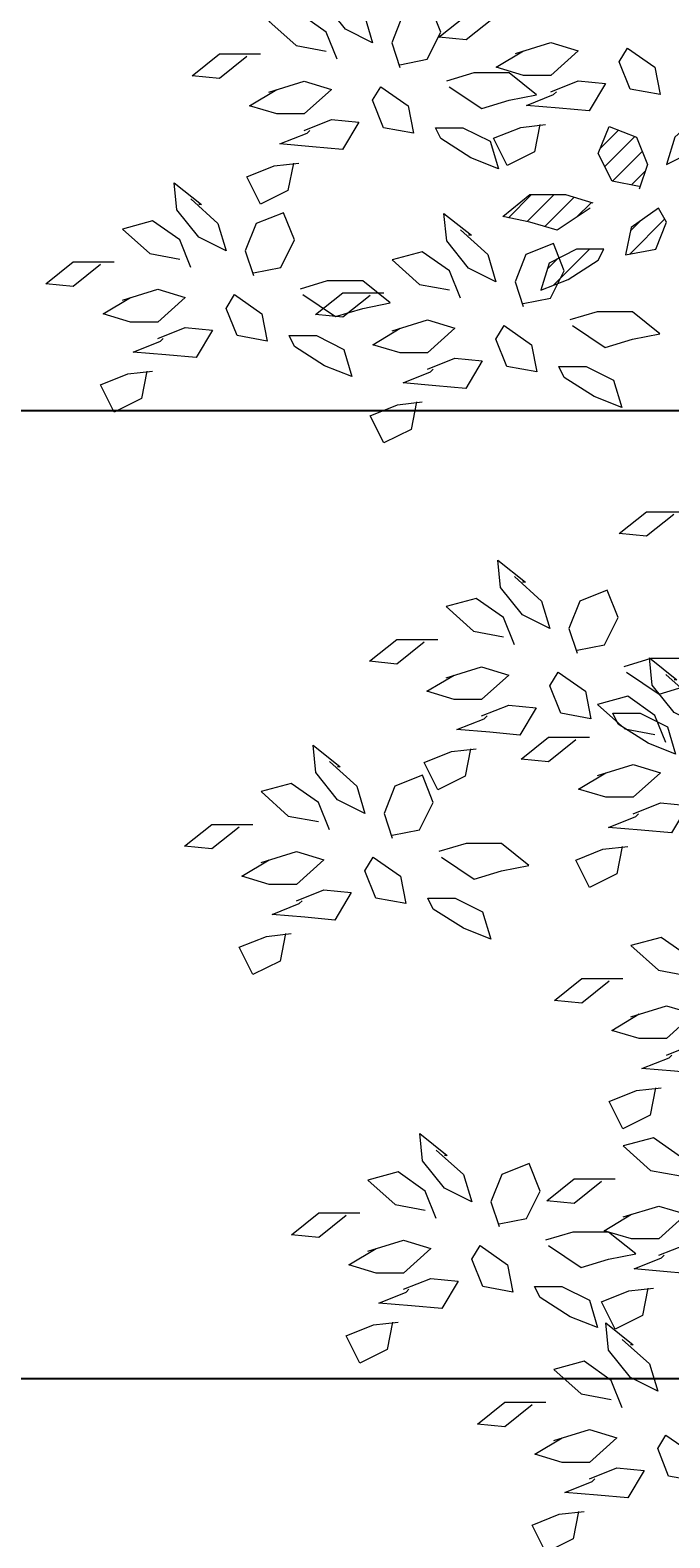
# Model space of a CAD drawing. Units: inches. Extents: x 1770 to 2988, y 1161 to 3221.
# Tile 39 of 44: x 2655 to 2687, y 2750 to 2825. Entities that reach past the tile are written whole.
import ezdxf

# ---------------------------------------------------------------- set-up
doc = ezdxf.new("R2010")
doc.units = ezdxf.units.IN
doc.layers.add('A-ANNO-DIMS', color=2, linetype='Continuous', lineweight=18)
doc.layers.add('trees1', color=250, linetype='Continuous', lineweight=13)
doc.styles.get("Standard").update_dxf_attribs({"font": 'arial.ttf'})
doc.dimstyles.get("Standard").update_dxf_attribs({"dimtxt": 0.18, "dimasz": 0.18, "dimexe": 0.18, "dimexo": 0.0625, "dimgap": 0.09, "dimtad": 0, "dimtih": 1, "dimtoh": 1, "dimdec": 4, "dimzin": 0, "dimdsep": 46, "dimtxsty": 'Standard', "dimcen": 0.09, "dimadec": 0, "dimazin": 0, "dimtfac": 1, "dimtdec": 4, "dimtofl": 0, "dimtmove": 0, "dimatfit": 3, "dimfxl": 1, "dimtolj": 1, "dimtzin": 0, "dimarcsym": 0})

# ---------------------------------------------------------------- blocks, each defined once
blk = doc.blocks.new('*X10')
at = {"color": 0}
for p, q in [((0.5118, -0.9024), (0.54, -0.8742)), ((0.5068, -0.8897), (0.5149, -0.8816))]:
    blk.add_line(p, q, dxfattribs=at)
blk = doc.blocks.new('*X11')
at = {"color": 0}
for p, q in [((0.5716, -0.8779), (0.5992, -0.8504)), ((0.5721, -0.8598), (0.5799, -0.852))]:
    blk.add_line(p, q, dxfattribs=at)
blk = doc.blocks.new('*X12')
at = {"color": 0}
for p, q in [((0.4764, -0.8494), (0.4945, -0.8313)), ((0.4911, -0.8524), (0.5122, -0.8313)), ((0.5049, -0.8563), (0.5279, -0.8333)), ((0.5296, -0.8493), (0.5415, -0.8374))]:
    blk.add_line(p, q, dxfattribs=at)
blk = doc.blocks.new('*X13')
at = {"color": 0}
for p, q in [((0.5486, -0.7949), (0.5629, -0.7806)), ((0.552, -0.8092), (0.5755, -0.7857)), ((0.5582, -0.8207), (0.5814, -0.7974)), ((0.5729, -0.8236), (0.5839, -0.8126))]:
    blk.add_line(p, q, dxfattribs=at)
blk = doc.blocks.new('tree342')
at = {"color": 0}
for points in [[(-770.6, 1840.1), (-749.1, 1820.8), (-742.7, 1799.4), (-764.1, 1810.1), (-781.3, 1831.6), (-783.5, 1853), (-762, 1835.8), (-764.1, 1835.8)], [(-721.2, 1782.2), (-699.7, 1786.5), (-689, 1807.9), (-697.6, 1829.4), (-719.1, 1820.8), (-727.6, 1799.4), (-721.2, 1780)], [(-770.6, 1786.5), (-779.2, 1807.9), (-800.7, 1823), (-824.3, 1816.5), (-802.8, 1797.2), (-779.2, 1792.9)], [(-647.7, 1818.9), (-669.2, 1801.7), (-690.7, 1803.9), (-669.2, 1821), (-637, 1821)], [(-841.5, 1788.6), (-862.9, 1771.5), (-884.4, 1773.6), (-862.9, 1790.8), (-830.7, 1790.8)], [(-630.5, 1791), (-602.6, 1799.6), (-581.1, 1793.1), (-602.6, 1773.8), (-624.1, 1773.8), (-645.6, 1780.3), (-624.1, 1793.1)], [(-824.3, 1760.7), (-796.4, 1769.3), (-774.9, 1762.9), (-796.4, 1743.6), (-817.8, 1743.6), (-839.3, 1750), (-817.8, 1762.9)], [(-682.5, 1765), (-656.8, 1747.9), (-635.3, 1754.3), (-613.8, 1758.6), (-635.3, 1775.8), (-663.2, 1775.8), (-684.7, 1769.3)], [(-602.6, 1760.9), (-581.1, 1769.5), (-559.7, 1767.4), (-572.5, 1745.9), (-596.2, 1748.1), (-621.9, 1750.2), (-600.5, 1758.8), (-598.3, 1760.9)], [(-483.8, 1744.6), (-505.2, 1725.3), (-511.7, 1703.8), (-490.2, 1714.5), (-473, 1736), (-470.9, 1757.5), (-492.4, 1740.3), (-490.2, 1740.3)], [(-796.4, 1730.7), (-774.9, 1739.3), (-753.4, 1737.1), (-766.3, 1715.7), (-789.9, 1717.8), (-815.7, 1720), (-794.2, 1728.5), (-792.1, 1730.7)], [(-611.2, 1735.2), (-615.5, 1713.7), (-637, 1703), (-647.7, 1724.5), (-626.2, 1733), (-606.9, 1735.2)], [(-533.2, 1686.6), (-554.6, 1690.9), (-565.4, 1712.4), (-556.8, 1733.8), (-535.3, 1725.3), (-526.7, 1703.8), (-533.2, 1684.5)], [(-804.9, 1704.9), (-809.2, 1683.5), (-830.7, 1672.7), (-841.5, 1694.2), (-820, 1702.8), (-800.7, 1704.9)], [(-885.6, 1676.8), (-864.2, 1657.5), (-857.7, 1636), (-879.2, 1646.7), (-896.4, 1668.2), (-898.5, 1689.6), (-877, 1672.5), (-879.2, 1672.5)], [(-571.8, 1669.5), (-597.6, 1652.3), (-619.1, 1658.7), (-640.5, 1663), (-619.1, 1680.2), (-591.1, 1680.2), (-569.7, 1673.8)], [(-885.6, 1623.1), (-894.2, 1644.6), (-915.7, 1659.6), (-939.3, 1653.2), (-917.8, 1633.9), (-894.2, 1629.6)], [(-836.2, 1618.8), (-814.8, 1623.1), (-804, 1644.6), (-812.6, 1666), (-834.1, 1657.5), (-842.7, 1636), (-836.2, 1616.7)], [(-673.7, 1652.6), (-652.2, 1633.3), (-645.8, 1611.8), (-667.3, 1622.5), (-684.5, 1644), (-686.6, 1665.4), (-665.1, 1648.3), (-667.3, 1648.3)], [(-673.7, 1598.9), (-682.3, 1620.4), (-703.8, 1635.4), (-727.4, 1629), (-705.9, 1609.6), (-682.3, 1605.4)], [(-624.3, 1594.6), (-602.9, 1598.9), (-592.1, 1620.4), (-600.7, 1641.8), (-622.2, 1633.3), (-630.8, 1611.8), (-624.3, 1592.5)], [(-956.5, 1625.3), (-978, 1608.1), (-999.4, 1610.2), (-978, 1627.4), (-945.8, 1627.4)], [(-797.6, 1601.7), (-771.8, 1584.5), (-750.3, 1590.9), (-728.9, 1595.2), (-750.3, 1612.4), (-778.3, 1612.4), (-799.7, 1606)], [(-939.3, 1597.4), (-911.4, 1606), (-889.9, 1599.5), (-911.4, 1580.2), (-932.9, 1580.2), (-954.3, 1586.6), (-932.9, 1599.5)], [(-744.6, 1601.1), (-766.1, 1583.9), (-787.5, 1586), (-766.1, 1603.2), (-733.8, 1603.2)], [(-585.7, 1577.5), (-559.9, 1560.3), (-538.4, 1566.7), (-517, 1571), (-538.4, 1588.2), (-566.3, 1588.2), (-587.8, 1581.8)], [(-911.4, 1567.3), (-889.9, 1575.9), (-868.4, 1573.8), (-881.3, 1552.3), (-905, 1554.4), (-930.7, 1556.6), (-909.2, 1565.2), (-907.1, 1567.3)], [(-727.4, 1573.2), (-699.5, 1581.8), (-678, 1575.3), (-699.5, 1556), (-721, 1556), (-742.4, 1562.4), (-721, 1575.3)], [(-699.5, 1543.1), (-678, 1551.7), (-656.5, 1549.6), (-669.4, 1528.1), (-693, 1530.2), (-718.8, 1532.4), (-697.3, 1541), (-695.2, 1543.1)], [(-920, 1541.6), (-924.3, 1520.1), (-945.8, 1509.4), (-956.5, 1530.8), (-935, 1539.4), (-915.7, 1541.6)], [(-708.1, 1517.4), (-712.4, 1495.9), (-733.8, 1485.2), (-744.6, 1506.6), (-723.1, 1515.2), (-703.8, 1517.4)], [(-506.1, 1429.1), (-527.6, 1411.9), (-549, 1414.1), (-527.6, 1431.2), (-495.4, 1431.2)], [(-631.3, 1380.3), (-609.9, 1361), (-603.4, 1339.5), (-624.9, 1350.3), (-642.1, 1371.7), (-644.2, 1393.2), (-622.7, 1376), (-624.9, 1376)], [(-631.3, 1326.6), (-639.9, 1348.1), (-661.4, 1363.1), (-685, 1356.7), (-663.5, 1337.4), (-639.9, 1333.1)], [(-581.9, 1322.4), (-560.5, 1326.6), (-549.7, 1348.1), (-558.3, 1369.6), (-579.8, 1361), (-588.4, 1339.5), (-581.9, 1320.2)], [(-702.2, 1328.8), (-723.7, 1311.6), (-745.1, 1313.8), (-723.7, 1330.9), (-691.5, 1330.9)], [(-543.3, 1305.2), (-517.5, 1288), (-496, 1294.5), (-474.6, 1298.7), (-496, 1315.9), (-524, 1315.9), (-545.4, 1309.5)], [(-512.3, 1303.5), (-490.8, 1284.2), (-484.3, 1262.8), (-505.8, 1273.5), (-523, 1294.9), (-525.1, 1316.4), (-503.7, 1299.2), (-505.8, 1299.2)], [(-685, 1300.9), (-657.1, 1309.5), (-635.6, 1303), (-657.1, 1283.7), (-678.6, 1283.7), (-700.1, 1290.2), (-678.6, 1303)], [(-657.1, 1270.9), (-635.6, 1279.4), (-614.2, 1277.3), (-627, 1255.8), (-650.7, 1258), (-676.4, 1260.1), (-655, 1268.7), (-652.8, 1270.9)], [(-512.3, 1249.9), (-520.9, 1271.3), (-542.3, 1286.4), (-566, 1279.9), (-544.5, 1260.6), (-520.9, 1256.3)], [(-776.6, 1235.1), (-755.2, 1215.8), (-748.7, 1194.3), (-770.2, 1205), (-787.4, 1226.5), (-789.5, 1248), (-768.1, 1230.8), (-770.2, 1230.8)], [(-665.7, 1245.1), (-670, 1223.6), (-691.5, 1212.9), (-702.2, 1234.4), (-680.7, 1243), (-661.4, 1245.1)], [(-583.1, 1252), (-604.6, 1234.9), (-626.1, 1237), (-604.6, 1254.2), (-572.4, 1254.2)], [(-566, 1224.1), (-538, 1232.7), (-516.6, 1226.3), (-538, 1207), (-559.5, 1207), (-581, 1213.4), (-559.5, 1226.3)], [(-727.3, 1177.1), (-705.8, 1181.4), (-695, 1202.9), (-703.6, 1224.4), (-725.1, 1215.8), (-733.7, 1194.3), (-727.3, 1175)], [(-776.6, 1181.4), (-785.2, 1202.9), (-806.7, 1217.9), (-830.3, 1211.5), (-808.9, 1192.2), (-785.2, 1187.9)], [(-538, 1194.1), (-516.6, 1202.7), (-495.1, 1200.5), (-508, 1179.1), (-531.6, 1181.2), (-557.4, 1183.3), (-535.9, 1191.9), (-533.7, 1194.1)], [(-847.5, 1183.6), (-869, 1166.4), (-890.5, 1168.6), (-869, 1185.7), (-836.8, 1185.7)], [(-830.3, 1155.7), (-802.4, 1164.3), (-780.9, 1157.8), (-802.4, 1138.5), (-823.9, 1138.5), (-845.4, 1145), (-823.9, 1157.8)], [(-688.6, 1160), (-662.8, 1142.8), (-641.4, 1149.2), (-619.9, 1153.5), (-641.4, 1170.7), (-669.3, 1170.7), (-690.7, 1164.3)], [(-546.6, 1168.3), (-550.9, 1146.9), (-572.4, 1136.1), (-583.1, 1157.6), (-561.7, 1166.2), (-542.3, 1168.3)], [(-802.4, 1125.6), (-780.9, 1134.2), (-759.5, 1132.1), (-772.3, 1110.6), (-796, 1112.8), (-821.7, 1114.9), (-800.3, 1123.5), (-798.1, 1125.6)], [(-811, 1099.9), (-815.3, 1078.4), (-836.8, 1067.7), (-847.5, 1089.2), (-826, 1097.7), (-806.7, 1099.9)], [(-486, 1060.4), (-494.6, 1081.9), (-516.1, 1096.9), (-539.7, 1090.5), (-518.2, 1071.2), (-494.6, 1066.9)], [(-556.9, 1062.6), (-578.4, 1045.4), (-599.8, 1047.5), (-578.4, 1064.7), (-546.2, 1064.7)], [(-539.7, 1034.7), (-511.8, 1043.3), (-490.3, 1036.8), (-511.8, 1017.5), (-533.3, 1017.5), (-554.7, 1023.9), (-533.3, 1036.8)], [(-511.8, 1004.6), (-490.3, 1013.2), (-468.8, 1011.1), (-481.7, 989.6), (-505.4, 991.8), (-531.1, 993.9), (-509.6, 1002.5), (-507.5, 1004.6)], [(-520.4, 978.9), (-524.7, 957.4), (-546.2, 946.7), (-556.9, 968.1), (-535.4, 976.7), (-516.1, 978.9)], [(-692.7, 930), (-671.2, 910.7), (-664.8, 889.2), (-686.2, 900), (-703.4, 921.4), (-705.6, 942.9), (-684.1, 925.7), (-686.2, 925.7)], [(-492.1, 903.1), (-500.7, 924.6), (-522.1, 939.6), (-545.8, 933.2), (-524.3, 913.8), (-500.7, 909.6)], [(-692.7, 876.3), (-701.3, 897.8), (-722.7, 912.8), (-746.4, 906.4), (-724.9, 887.1), (-701.3, 882.8)], [(-643.3, 872.1), (-621.8, 876.3), (-611.1, 897.8), (-619.7, 919.3), (-641.1, 910.7), (-649.7, 889.2), (-643.3, 869.9)], [(-562.9, 905.3), (-584.4, 888.1), (-605.9, 890.2), (-584.4, 907.4), (-552.2, 907.4)], [(-763.5, 878.5), (-785, 861.3), (-806.5, 863.5), (-785, 880.6), (-752.8, 880.6)], [(-545.8, 877.4), (-517.8, 885.9), (-496.4, 879.5), (-517.8, 860.2), (-539.3, 860.2), (-560.8, 866.6), (-539.3, 879.5)], [(-604.6, 854.9), (-578.9, 837.7), (-557.4, 844.2), (-535.9, 848.5), (-557.4, 865.6), (-585.3, 865.6), (-606.8, 859.2)], [(-746.4, 850.6), (-718.4, 859.2), (-697, 852.7), (-718.4, 833.4), (-739.9, 833.4), (-761.4, 839.9), (-739.9, 852.7)], [(-517.8, 847.3), (-496.4, 855.9), (-474.9, 853.8), (-487.8, 832.3), (-511.4, 834.4), (-537.2, 836.6), (-515.7, 845.2), (-513.6, 847.3)], [(-718.4, 820.6), (-697, 829.1), (-675.5, 827), (-688.4, 805.5), (-712, 807.7), (-737.8, 809.8), (-716.3, 818.4), (-714.1, 820.6)], [(-526.4, 821.6), (-530.7, 800.1), (-552.2, 789.4), (-562.9, 810.8), (-541.5, 819.4), (-522.1, 821.6)], [(-727, 794.8), (-731.3, 773.3), (-752.8, 762.6), (-763.5, 784.1), (-742.1, 792.7), (-722.7, 794.8)], [(-546.6, 781.3), (-525.1, 762), (-518.7, 740.5), (-540.1, 751.3), (-557.3, 772.7), (-559.5, 794.2), (-538, 777), (-540.1, 777)], [(-546.6, 727.6), (-555.2, 749.1), (-576.6, 764.1), (-600.3, 757.7), (-578.8, 738.4), (-555.2, 734.1)], [(-617.4, 729.8), (-638.9, 712.6), (-660.4, 714.8), (-638.9, 731.9), (-606.7, 731.9)], [(-600.3, 701.9), (-572.3, 710.5), (-550.9, 704), (-572.3, 684.7), (-593.8, 684.7), (-615.3, 691.2), (-593.8, 704)], [(-572.3, 671.9), (-550.9, 680.4), (-529.4, 678.3), (-542.3, 656.8), (-565.9, 659), (-591.7, 661.1), (-570.2, 669.7), (-568, 671.9)], [(-580.9, 646.1), (-585.2, 624.6), (-606.7, 613.9), (-617.4, 635.4), (-596, 644), (-576.6, 646.1)]]:
    blk.add_lwpolyline(points, dxfattribs=at)
for points in [[(-521, 1780.3), (-516.7, 1758.8), (-540.3, 1763.1), (-548.9, 1784.5), (-542.5, 1795.3)], [(-714.8, 1750), (-710.5, 1728.5), (-734.1, 1732.8), (-742.7, 1754.3), (-736.2, 1765)], [(-671.8, 1732.8), (-650.3, 1722.1), (-643.9, 1700.6), (-665.4, 1709.2), (-689, 1724.3), (-693.3, 1732.8)], [(-539.6, 1654.4), (-543.9, 1633), (-520.3, 1637.3), (-511.7, 1658.7), (-518.1, 1669.5)], [(-582.5, 1637.3), (-604, 1626.5), (-610.5, 1605.1), (-589, 1613.7), (-565.4, 1628.7), (-561.1, 1637.3)], [(-829.8, 1586.6), (-825.5, 1565.2), (-849.1, 1569.5), (-857.7, 1590.9), (-851.3, 1601.7)], [(-617.9, 1562.4), (-613.6, 1541), (-637.2, 1545.3), (-645.8, 1566.7), (-639.4, 1577.5)], [(-786.8, 1569.5), (-765.4, 1558.7), (-758.9, 1537.3), (-780.4, 1545.9), (-804, 1560.9), (-808.3, 1569.5)], [(-574.9, 1545.3), (-553.5, 1534.5), (-547, 1513.1), (-568.5, 1521.7), (-592.1, 1536.7), (-596.4, 1545.3)], [(-575.5, 1290.2), (-571.2, 1268.7), (-594.8, 1273), (-603.4, 1294.5), (-597, 1305.2)], [(-532.6, 1273), (-511.1, 1262.3), (-504.6, 1240.8), (-526.1, 1249.4), (-549.7, 1264.4), (-554, 1273)], [(-720.8, 1145), (-716.5, 1123.5), (-740.1, 1127.8), (-748.7, 1149.2), (-742.3, 1160)], [(-677.9, 1127.8), (-656.4, 1117.1), (-649.9, 1095.6), (-671.4, 1104.2), (-695, 1119.2), (-699.3, 1127.8)], [(-636.8, 839.9), (-632.5, 818.4), (-656.2, 822.7), (-664.8, 844.2), (-658.3, 854.9)], [(-593.9, 822.7), (-572.4, 812), (-566, 790.5), (-587.4, 799.1), (-611.1, 814.1), (-615.4, 822.7)], [(-490.7, 691.2), (-486.4, 669.7), (-510.1, 674), (-518.7, 695.5), (-512.2, 706.2)]]:
    blk.add_lwpolyline(points, close=True, dxfattribs=at)
at = {"color": 0, "xscale": 1000, "yscale": 1000, "zscale": 1000}
for name in ['*X13', '*X12', '*X11', '*X10']:
    blk.add_blockref(name, (-1112.3, 2511.5), dxfattribs=at)
blk = doc.blocks.new('*D96')
at = {"layer": 'A-ANNO-DIMS', "color": 0, "lineweight": -2, "transparency": 16777216}
for p, q in [((2620.113, 2758.297), (2801.915, 2758.297)), ((2801.735, 2758.117), (2801.735, 2740.479)), ((2801.735, 2722.477), (2801.735, 2740.115)), ((2655.505, 2722.297), (2801.915, 2722.297))]:
    blk.add_line(p, q, dxfattribs=at)
at = {"layer": 'A-ANNO-DIMS', "color": 0, "transparency": 16777216}
for points in [[(2801.705, 2758.117), (2801.765, 2758.117), (2801.735, 2758.297)], [(2801.705, 2722.477), (2801.765, 2722.477), (2801.735, 2722.297)]]:
    blk.add_solid(points, dxfattribs=at)
at = {"layer": 'Defpoints', "color": 0, "transparency": 16777216}
for p in [(2620.051, 2758.297), (2801.735, 2758.297), (2655.443, 2722.297)]:
    blk.add_point(p, dxfattribs=at)
at = {"layer": 'A-ANNO-DIMS', "color": 0, "transparency": 16777216, "insert": (2801.735, 2740.297), "char_height": 0.18, "attachment_point": 5}
blk.add_mtext('\\A1;36', dxfattribs=at)
blk = doc.blocks.new('*D97')
at = {"layer": 'A-ANNO-DIMS', "color": 0, "lineweight": -2, "transparency": 16777216}
for p, q in [((2620.113, 2806.297), (2801.915, 2806.297)), ((2801.735, 2806.117), (2801.735, 2782.479)), ((2801.735, 2758.477), (2801.735, 2782.115)), ((2620.113, 2758.297), (2801.915, 2758.297))]:
    blk.add_line(p, q, dxfattribs=at)
at = {"layer": 'A-ANNO-DIMS', "color": 0, "transparency": 16777216}
for points in [[(2801.705, 2806.117), (2801.765, 2806.117), (2801.735, 2806.297)], [(2801.705, 2758.477), (2801.765, 2758.477), (2801.735, 2758.297)]]:
    blk.add_solid(points, dxfattribs=at)
at = {"layer": 'Defpoints', "color": 0, "transparency": 16777216}
for p in [(2620.051, 2806.297), (2801.735, 2806.297), (2620.051, 2758.297)]:
    blk.add_point(p, dxfattribs=at)
at = {"layer": 'A-ANNO-DIMS', "color": 0, "transparency": 16777216, "insert": (2801.735, 2782.297), "char_height": 0.18, "attachment_point": 5}
blk.add_mtext('\\A1;48', dxfattribs=at)
blk = doc.blocks.new('*D98')
at = {"layer": 'A-ANNO-DIMS', "color": 0, "lineweight": -2, "transparency": 16777216}
for p, q in [((2655.505, 2842.297), (2801.915, 2842.297)), ((2801.735, 2842.117), (2801.735, 2824.479)), ((2801.735, 2806.477), (2801.735, 2824.115)), ((2620.113, 2806.297), (2801.915, 2806.297))]:
    blk.add_line(p, q, dxfattribs=at)
at = {"layer": 'A-ANNO-DIMS', "color": 0, "transparency": 16777216}
for points in [[(2801.705, 2842.117), (2801.765, 2842.117), (2801.735, 2842.297)], [(2801.705, 2806.477), (2801.765, 2806.477), (2801.735, 2806.297)]]:
    blk.add_solid(points, dxfattribs=at)
at = {"layer": 'Defpoints', "color": 0, "transparency": 16777216}
for p in [(2655.443, 2842.297), (2801.735, 2842.297), (2620.051, 2806.297)]:
    blk.add_point(p, dxfattribs=at)
at = {"layer": 'A-ANNO-DIMS', "color": 0, "transparency": 16777216, "insert": (2801.735, 2824.297), "char_height": 0.18, "attachment_point": 5}
blk.add_mtext('\\A1;36', dxfattribs=at)

msp = doc.modelspace()

# ---------------------------------------------------------------- block references
at = {"layer": 'trees1', "xscale": 0.063143750371755, "yscale": 0.063143750371755, "zscale": 0.063143750371755}
msp.add_blockref('tree342', (2719.3275, 2710.8976), dxfattribs=at)

# ---------------------------------------------------------------- dimensions: what is measured, and where the dimension line sits
at = {"layer": 'A-ANNO-DIMS'}
for base, p1, p2, picture, middle in [((2801.7346, 2842.2969), (2620.0508, 2806.2969), (2655.443, 2842.2969), '*D98', (2801.7346, 2824.2969)), ((2801.7346, 2806.2969), (2620.0508, 2758.2969), (2620.0508, 2806.2969), '*D97', (2801.7346, 2782.2969)), ((2801.7346, 2758.2969), (2655.443, 2722.2969), (2620.0508, 2758.2969), '*D96', (2801.7346, 2740.2969))]:
    dim = msp.add_linear_dim(base=base, p1=p1, p2=p2, angle=90, dimstyle='Standard', override={"dimdec": 0, "dimlfac": 1, "dimrnd": 0, "dimzin": 0, "dimdsep": 46, "dimlunit": 2}, dxfattribs=at)
    dim.commit()
    dim.dimension.update_dxf_attribs({"geometry": picture, "text_midpoint": middle})

doc.saveas('drawing.dxf')
